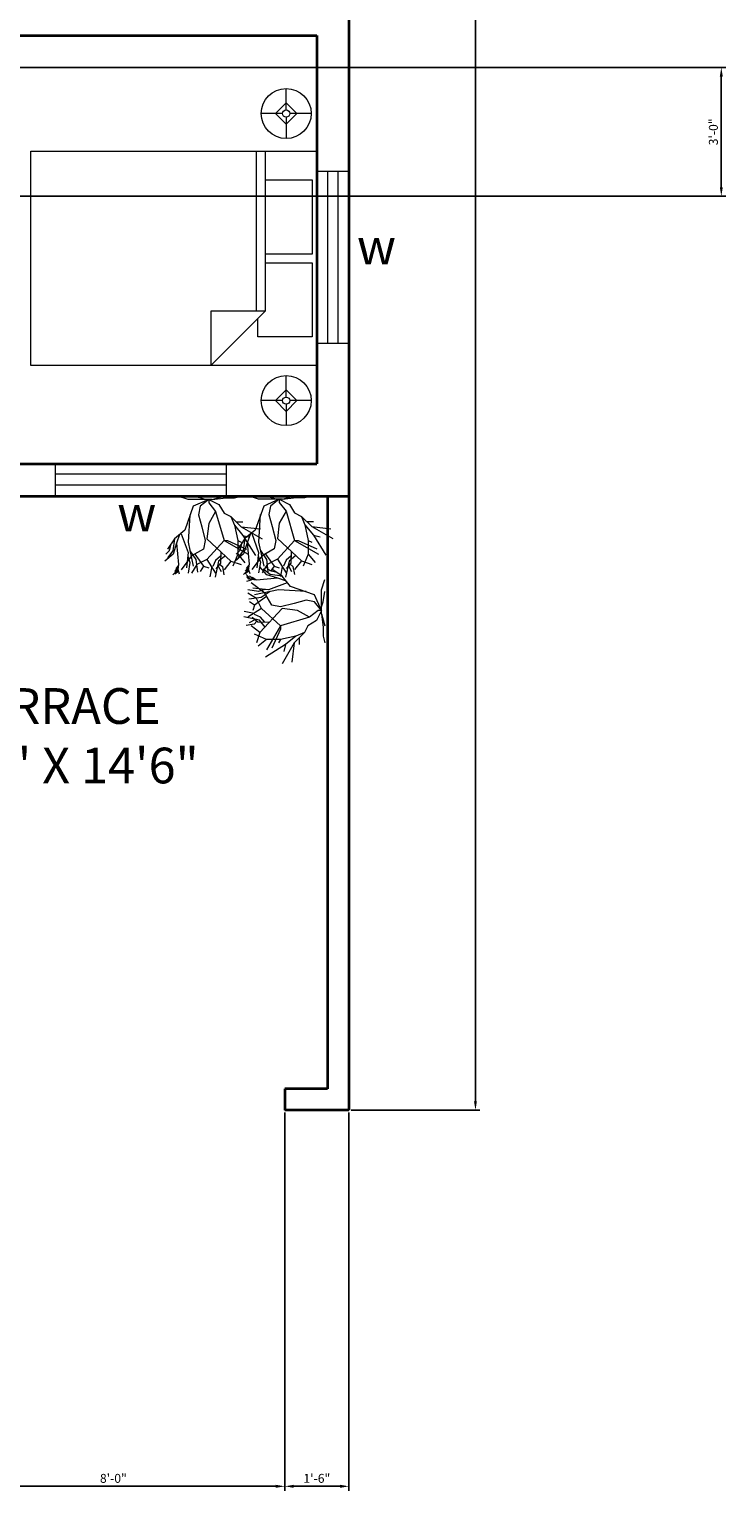
# Model space of a CAD drawing. Units: inches. Extents: x 2729 to 3178, y 5006 to 5809.
# Tile 2 of 4: x 2983 to 3178, y 5006 to 5415. Entities that reach past the tile are written whole.
import ezdxf

# ---------------------------------------------------------------- set-up
doc = ezdxf.new("R2010")
doc.units = ezdxf.units.IN
doc.layers.get('Defpoints').update_dxf_attribs({"color": 72})
for name, color, linetype, lineweight in [('A-ANNO-DIMS', 2, 'Continuous', 18), ('A-ANNO-TEXT', 7, 'Continuous', 18), ('A-AREA-IDEN', 7, 'Continuous', 25), ('A-FURN', 8, 'Continuous', 18), ('A-GLAZ', 4, 'Continuous', 18), ('A-WALL', 7, 'Continuous', 35), ('L-PLNT', 72, 'Continuous', 13)]:
    doc.layers.add(name, color=color, linetype=linetype, lineweight=lineweight)
doc.styles.get("Standard").update_dxf_attribs({"font": 'arial.ttf'})
doc.dimstyles.new('ISO-25', dxfattribs={"dimtxt": 2.5, "dimasz": 2.5, "dimexe": 1.25, "dimexo": 0.625, "dimtad": 1, "dimdec": 0, "dimlunit": 3, "dimtxsty": 'Standard', "dimcen": 2.5, "dimadec": 0, "dimazin": 0, "dimtfac": 1, "dimtdec": 0, "dimtmove": 0, "dimatfit": 3, "dimfxl": 1, "dimarcsym": 0})

# ---------------------------------------------------------------- blocks, each defined once
blk = doc.blocks.new('*D2')
at = {"layer": 'A-ANNO-DIMS', "color": 0, "lineweight": -2, "transparency": 16777216}
for p, q in [((3072.8, 5760.64), (3108.86, 5760.64)), ((3107.61, 5758.14), (3107.61, 5115.14)), ((3072.8, 5112.64), (3108.86, 5112.64))]:
    blk.add_line(p, q, dxfattribs=at)
at = {"layer": 'A-ANNO-DIMS', "color": 0, "transparency": 16777216}
for points in [[(3107.19, 5758.14), (3108.02, 5758.14), (3107.61, 5760.64)], [(3107.19, 5115.14), (3108.02, 5115.14), (3107.61, 5112.64)]]:
    blk.add_solid(points, dxfattribs=at)
at = {"layer": 'Defpoints', "color": 0, "transparency": 16777216}
for p in [(3072.18, 5760.64), (3072.18, 5112.64), (3107.61, 5112.64)]:
    blk.add_point(p, dxfattribs=at)
at = {"layer": 'A-ANNO-DIMS', "color": 0, "transparency": 16777216, "insert": (3101.9, 5436.64), "char_height": 2.5, "attachment_point": 5, "rotation": 90}
blk.add_mtext("{\\H4x;54'}", dxfattribs=at)
blk = doc.blocks.new('Bed - Queen')
for p, q in [((0, -80.00003), (0, 0)), ((0, 0), (59.99999, 0)), ((59.99999, 0), (59.99999, -80.00003)), ((7.99999, -1.2), (28.79998, -1.2)), ((7.99999, -14.4), (7.99999, -1.2)), ((28.79998, -1.2), (28.79998, -14.4)), ((31.19999, -1.2), (51.99999, -1.2)), ((31.19999, -14.4), (31.19999, -1.2)), ((51.99999, -1.2), (51.99999, -16.4)), ((0, -14.4), (44.8, -14.4)), ((59.99999, -29.6), (44.8, -14.4)), ((44.8, -14.4), (44.8, -29.6)), ((44.8, -16.8), (0, -16.8)), ((51.99999, -16.4), (46.79936, -16.4)), ((44.8, -29.6), (59.99999, -29.6)), ((59.99999, -80.00003), (0, -80.00003))]:
    blk.add_line(p, q)
blk = doc.blocks.new('Lamp - Table')
for p, q in [((0, 7), (0, 1)), ((-1, 0), (-7, 0)), ((0, 3), (-3, 0)), ((-3, 0), (0, -3)), ((3, 0), (0, 3)), ((0, -3), (3, 0)), ((1, 0), (7, 0)), ((0, -1), (0, -7))]:
    blk.add_line(p, q)
for radius in [7, 1]:
    blk.add_circle((0, 0), radius)
blk = doc.blocks.new('*U13')
for p, q in [((-377.952, 463.296), (-329.184, 524.256)), ((-316.7634, 502.285), (-327.6092, 559.9176)), ((-286.512, 498.3226), (-307.4416, 538.0736)), ((-290.3982, 464.5406), (-265.6078, 577.8246)), ((-207.264, 451.104), (-268.224, 548.64)), ((-240.792, 502.285), (-228.3968, 573.8368)), ((-182.88, 499.872), (-158.496, 536.448)), ((-129.1844, 450.6214), (-140.0302, 542.036)), ((-134.112, 487.68), (-97.536, 548.64)), ((-97.536, 426.72), (-24.384, 524.256)), ((-85.7758, 472.4908), (-73.3552, 548.005)), ((-12.9032, 555.9552), (-2.0574, 522.1732)), ((-5.1562, 486.3846), (2.5908, 542.036)), ((-0.508, 508.254), (22.7584, 536.067)), ((1.0414, 526.1356), (35.1536, 559.9176)), ((2.5908, 542.036), (21.209, 555.9552)), ((-463.296, 280.416), (-552.577, 423.037)), ((-426.72, 414.528), (-475.488, 475.488)), ((-377.952, 463.296), (-451.104, 487.68)), ((-426.72, 414.528), (-390.144, 499.872)), ((-207.264, 304.8), (-377.952, 463.296)), ((-338.455, 424.7896), (-290.3982, 464.5406)), ((-329.184, 316.992), (-207.264, 451.104)), ((-296.5958, 484.4034), (-316.7634, 502.285)), ((-305.8922, 396.9512), (-302.7934, 478.4344)), ((-304.3428, 426.7708), (-268.7066, 458.5716)), ((-302.7934, 478.4344), (-270.256, 518.1854)), ((-268.7066, 458.5716), (-250.0884, 500.3038)), ((-182.88, 499.872), (-219.456, 512.064)), ((-207.264, 451.104), (-134.112, 487.68)), ((-121.92, 414.528), (-182.88, 499.872)), ((-182.88, 377.952), (-97.536, 426.72)), ((-85.7758, 389.001), (-129.1844, 452.6026)), ((-73.152, 329.184), (-109.728, 499.872)), ((-70.2564, 426.7708), (-85.7758, 472.4908)), ((-73.152, 402.336), (-60.96, 512.064)), ((8.7884, 335.3562), (-5.1562, 486.3846)), ((-3.6068, 492.3536), (14.986, 518.1854)), ((33.6042, 412.8516), (92.5068, 464.5406)), ((36.576, 390.144), (73.152, 438.912)), ((-329.184, 316.992), (-499.872, 414.528)), ((-353.568, 316.992), (-487.68, 377.952)), ((-426.72, 316.992), (-451.104, 329.184)), ((-426.72, 316.992), (-426.72, 414.528)), ((-402.336, 207.264), (-426.72, 316.992)), ((-329.184, 316.992), (-353.568, 316.992)), ((-268.224, 109.728), (-329.184, 316.992)), ((-195.072, 316.992), (-182.88, 377.952)), ((-170.688, 219.456), (-195.072, 316.992)), ((-85.344, 134.112), (-73.152, 329.184)), ((-24.384, 268.224), (-73.152, 402.336)), ((-12.192, 274.32), (8.7884, 335.3562)), ((8.7884, 335.3562), (33.6042, 412.8516)), ((24.384, 304.8), (36.576, 390.144)), ((24.384, 304.8), (73.152, 377.952)), ((48.768, 341.376), (60.96, 390.144)), ((60.96, 390.144), (85.344, 414.528)), ((-451.104, 219.456), (-601.0402, 303.8094)), ((-451.104, 219.456), (-587.4512, 234.2388)), ((-463.296, 280.416), (-512.064, 292.608)), ((-402.336, 207.264), (-463.296, 280.416)), ((-377.952, 146.304), (-451.104, 219.456)), ((-219.456, 195.072), (-207.264, 304.8)), ((-146.304, 134.112), (-170.688, 219.456)), ((-109.728, 73.152), (-48.768, 243.84)), ((-48.768, 243.84), (24.384, 304.8)), ((-414.528, 182.88), (-463.296, 182.88)), ((-377.952, 146.304), (-402.336, 207.264)), ((-329.184, 121.92), (-377.952, 146.304)), ((-292.608, 60.96), (-329.184, 121.92)), ((-268.224, 109.728), (-219.456, 195.072)), ((-219.456, 48.768), (-268.224, 109.728)), ((-158.496, 73.152), (-146.304, 134.112)), ((-402.336, 12.192), (-451.104, 0)), ((-341.376, 12.192), (-402.336, 12.192)), ((-243.84, 24.384), (-341.376, 12.192)), ((-243.84, 24.384), (-329.184, 0)), ((-219.456, 24.384), (-292.608, 60.96)), ((-243.84, 24.384), (-195.072, 24.384)), ((-219.456, 24.384), (-109.728, 73.152)), ((-219.456, 24.384), (-158.496, 73.152)), ((-219.456, 24.384), (-219.456, 48.768)), ((-219.456, 24.384), (-73.152, 24.384)), ((-195.072, 24.384), (-158.496, 12.192)), ((-158.496, 12.192), (-85.344, 0)), ((-73.152, 24.384), (0, 0))]:
    blk.add_line(p, q)
blk = doc.blocks.new('WIN-48IN')
for p, q in [((48, 9), (0, 9)), ((0, 9), (0, 0)), ((48, 0), (48, 9)), ((48, 6), (0, 6)), ((0, 3), (48, 3)), ((0, 0), (48, 0))]:
    blk.add_line(p, q)
blk = doc.blocks.new('*D51')
at = {"layer": 'A-ANNO-DIMS', "color": 0, "lineweight": -2, "transparency": 16777216}
for p, q in [((2958.18, 5112.01), (2958.18, 5006.05)), ((3054.18, 5112.01), (3054.18, 5006.05)), ((2960.68, 5007.3), (3051.68, 5007.3))]:
    blk.add_line(p, q, dxfattribs=at)
at = {"layer": 'A-ANNO-DIMS', "color": 0, "transparency": 16777216}
for points in [[(2960.68, 5007.72), (2960.68, 5006.88), (2958.18, 5007.3)], [(3051.68, 5007.72), (3051.68, 5006.88), (3054.18, 5007.3)]]:
    blk.add_solid(points, dxfattribs=at)
at = {"layer": 'Defpoints', "color": 0, "transparency": 16777216}
for p in [(2958.18, 5112.64), (3054.18, 5112.64), (3054.18, 5007.3)]:
    blk.add_point(p, dxfattribs=at)
at = {"layer": 'A-ANNO-DIMS', "color": 0, "transparency": 16777216, "insert": (3006.18, 5009.2), "char_height": 2.5, "attachment_point": 5}
blk.add_mtext('8\'-0"', dxfattribs=at)
blk = doc.blocks.new('*D52')
at = {"layer": 'A-ANNO-DIMS', "color": 0, "lineweight": -2, "transparency": 16777216}
for p, q in [((3054.18, 5112.01), (3054.18, 5006.05)), ((3072.18, 5112.01), (3072.18, 5006.05)), ((3056.68, 5007.3), (3069.68, 5007.3))]:
    blk.add_line(p, q, dxfattribs=at)
at = {"layer": 'A-ANNO-DIMS', "color": 0, "transparency": 16777216}
for points in [[(3056.68, 5007.72), (3056.68, 5006.88), (3054.18, 5007.3)], [(3069.68, 5007.72), (3069.68, 5006.88), (3072.18, 5007.3)]]:
    blk.add_solid(points, dxfattribs=at)
at = {"layer": 'Defpoints', "color": 0, "transparency": 16777216}
for p in [(3054.18, 5112.64), (3072.18, 5112.64), (3072.18, 5007.3)]:
    blk.add_point(p, dxfattribs=at)
at = {"layer": 'A-ANNO-DIMS', "color": 0, "transparency": 16777216, "insert": (3063.18, 5009.2), "char_height": 2.5, "attachment_point": 5}
blk.add_mtext('1\'-6"', dxfattribs=at)
blk = doc.blocks.new('*D53')
at = {"layer": 'A-ANNO-DIMS', "color": 0, "lineweight": -2, "transparency": 16777216}
for p, q in [((2838.8, 5404.64), (3177.73, 5404.64)), ((3176.48, 5371.14), (3176.48, 5402.14)), ((2838.8, 5368.64), (3177.73, 5368.64))]:
    blk.add_line(p, q, dxfattribs=at)
at = {"layer": 'A-ANNO-DIMS', "color": 0, "transparency": 16777216}
for points in [[(3176.06, 5402.14), (3176.9, 5402.14), (3176.48, 5404.64)], [(3176.06, 5371.14), (3176.9, 5371.14), (3176.48, 5368.64)]]:
    blk.add_solid(points, dxfattribs=at)
at = {"layer": 'Defpoints', "color": 0, "transparency": 16777216}
for p in [(2838.18, 5404.64), (3176.48, 5404.64), (2838.18, 5368.64)]:
    blk.add_point(p, dxfattribs=at)
at = {"layer": 'A-ANNO-DIMS', "color": 0, "transparency": 16777216, "insert": (3174.58, 5386.64), "char_height": 2.5, "attachment_point": 5, "rotation": 90}
blk.add_mtext('3\'-0"', dxfattribs=at)

msp = doc.modelspace()

# ---------------------------------------------------------------- linework, layer by layer
at = {"layer": 'A-WALL'}
for p, q in [((3072.18, 5760.64), (3072.18, 5112.64)), ((3072.18, 5760.64), (3072.18, 5112.64)), ((2916.18, 5413.64), (3063.18, 5413.64)), ((3063.18, 5413.64), (3063.18, 5293.64)), ((3063.18, 5413.64), (3063.18, 5293.64)), ((2958.18, 5293.64), (3063.18, 5293.64)), ((2958.18, 5284.64), (3063.18, 5284.64)), ((3063.18, 5284.64), (3072.18, 5284.64)), ((3066.18, 5284.64), (3066.18, 5118.64)), ((3066.18, 5118.64), (3054.18, 5118.64)), ((3066.18, 5118.64), (3054.18, 5118.64)), ((3054.18, 5118.64), (3054.18, 5112.64)), ((3072.18, 5112.64), (3054.18, 5112.64))]:
    msp.add_line(p, q, dxfattribs=at)

# ---------------------------------------------------------------- block references
at = {"layer": 'A-FURN', "rotation": 270}
for name, p in [('Lamp - Table', (3054.59, 5391.77)), ('Bed - Queen', (3063.09, 5381.2)), ('Lamp - Table', (3054.59, 5311.36))]:
    msp.add_blockref(name, p, dxfattribs=at)
at = {"layer": 'A-GLAZ', "rotation": 90.00000000000003}
msp.add_blockref('WIN-48IN', (3072.12, 5327.49), dxfattribs=at)
at = {"layer": 'A-GLAZ'}
msp.add_blockref('WIN-48IN', (2989.86, 5284.74), dxfattribs=at)
at = {"layer": 'L-PLNT', "xscale": 0.0393700787401575, "yscale": 0.0393700787401575, "zscale": 0.0393700787401575}
for p, rotation in [((3024.24, 5284.65), 180), ((3043.98, 5284.71), 180), ((3065.44, 5261.27), 90)]:
    msp.add_blockref('*U13', p, dxfattribs=dict(at, rotation=rotation))

# ---------------------------------------------------------------- texts
at = {"layer": 'A-ANNO-TEXT', "char_height": 10, "attachment_point": 1}
for insert in [(3074.41, 5359.52), (3007.26, 5284.74)]:
    msp.add_mtext_dynamic_manual_height_columns('w', width=11.1436, gutter_width=12.5, heights=[0], dxfattribs=dict(at, insert=insert))
at = {"layer": 'A-AREA-IDEN', "insert": (2938.41, 5230.84), "char_height": 10, "attachment_point": 1}
msp.add_mtext_dynamic_manual_height_columns('\\pxqc;TERRACE\\P12\'3" X 14\'6"', width=103.4579, gutter_width=12.5, heights=[0], dxfattribs=at)

# ---------------------------------------------------------------- dimensions: what is measured, and where the dimension line sits
at = {"layer": 'A-ANNO-DIMS'}
dim = msp.add_linear_dim(base=(3107.61, 5112.64), p1=(3072.18, 5760.64), p2=(3072.18, 5112.64), angle=90, text="{\\H4x;54'}", dimstyle='ISO-25', override={"dimclrd": 0, "dimclre": 0, "dimclrt": 0}, dxfattribs=at)
dim.commit()
dim.dimension.update_dxf_attribs({"geometry": '*D2', "text_midpoint": (3101.9, 5436.64)})
dim = msp.add_linear_dim(base=(3176.48, 5404.64), p1=(2838.18, 5368.64), p2=(2838.18, 5404.64), angle=90, dimstyle='ISO-25', override={"dimdec": 1, "dimlfac": 1, "dimrnd": 0, "dimzin": 1, "dimdsep": 46, "dimlunit": 4, "dimfrac": 2}, dxfattribs=at)
dim.commit()
dim.dimension.update_dxf_attribs({"geometry": '*D53', "text_midpoint": (3174.58, 5386.64)})
for base, p1, p2, picture, middle in [((3054.18, 5007.3), (2958.18, 5112.64), (3054.18, 5112.64), '*D51', (3006.18, 5009.2)), ((3072.18, 5007.3), (3054.18, 5112.64), (3072.18, 5112.64), '*D52', (3063.18, 5009.2))]:
    dim = msp.add_linear_dim(base=base, p1=p1, p2=p2, dimstyle='ISO-25', override={"dimdec": 1, "dimlfac": 1, "dimrnd": 0, "dimzin": 1, "dimdsep": 46, "dimlunit": 4, "dimfrac": 2}, dxfattribs=at)
    dim.commit()
    dim.dimension.update_dxf_attribs({"geometry": picture, "text_midpoint": middle})

doc.saveas('drawing.dxf')
